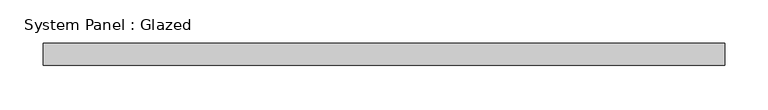
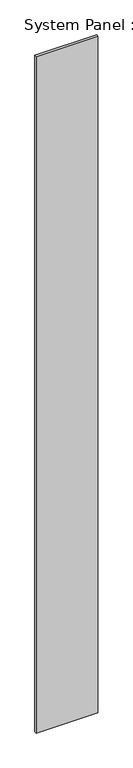
"""IFC4 building model written with IfcOpenShell, lengths in millimetres: plate geometry, System Panel : Glazed."""

from ifc_helpers import new_model, si_unit, origin, origin_with_axes, place, context, project, spatial, polyline, outline, extrude, source, transform, mapped, element, save


def system_panel_glazed_7e4c53f5(model_context):
    return source(origin(), model_context, "Body", "SweptSolid", [
        extrude(outline(polyline([(394.8155058, 19.05), (-394.8155058, 19.05), (-394.8155058, 44.45), (394.8155058, 44.45), (394.8155058, 19.05)])), origin_with_axes(), (0.0, 0.0, 1.0), 9144.0),
    ])


if __name__ == "__main__":
    model = new_model("IFC4")
    model_context = context("Model", 3, world=origin())
    ifc_project = project(units=[si_unit("LENGTHUNIT", "METRE", prefix="MILLI")], contexts=[model_context])
    site = spatial("IfcSite", under=ifc_project)
    building = spatial("IfcBuilding", under=site)
    placement = place(None, origin())
    system_panel_glazed_shape = system_panel_glazed_7e4c53f5(model_context)
    element("IfcPlate", 1, ObjectType="System Panel : Glazed", at=placement, inside=building, context=model_context, shape_type="MappedRepresentation", body=[
        mapped(system_panel_glazed_shape, transform((0.0, 0.0, 0.0), x_axis=(1.0, 0.0, 0.0), y_axis=(0.0, 1.0, 0.0), z_axis=(0.0, 0.0, 1.0))),
    ])
    save(model, "model.ifc")

# Revit data of these elements
# Type "System Panel : Glazed"
#   Construction Type Id = "GSP4R"
#   Analytic Construction = "1/8 in Pilkington single glazing"
#   Visual Light Transmittance = 0.9
#   Solar Heat Gain Coefficient = 0.86
#   Heat Transfer Coefficient (U) = 1.18115 BTU/(h·ft²·°F)
#   Define Thermal Properties by = 1
# Element 1 (IfcPlate, "System Panel : Glazed")
#   Materials on its faces: "Glass"
# Materials
#   "Glass": class "Glass", colour RGB 0 128 192, transparency 0.75, Description = "Soda Lime Glass", Cost = 0
